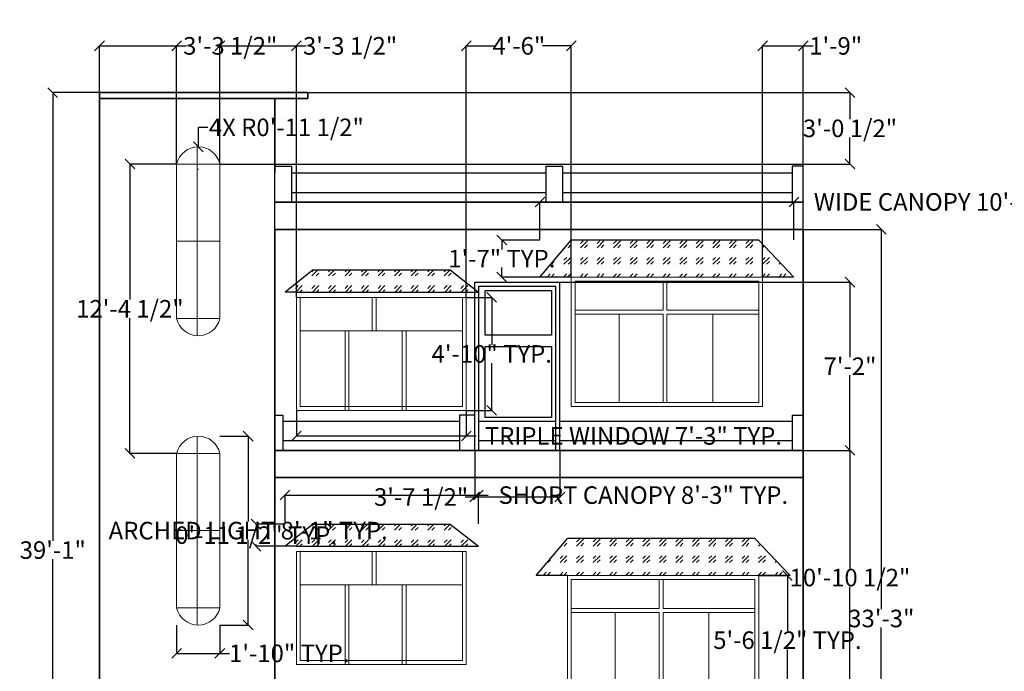
# Model space of a CAD drawing. Units: inches. Extents: x -19 to 1000, y -122 to 1144.
# Tile 7 of 8: x -19 to 486, y 501 to 835. Entities that reach past the tile are written whole.
import ezdxf

# ---------------------------------------------------------------- set-up
doc = ezdxf.new("R2010")
doc.units = ezdxf.units.IN
doc.header["$MEASUREMENT"] = 0
for name, color, linetype, lineweight in [('A-ANNO-DIMS', 191, 'Continuous', 18), ('A-ELEV', 4, 'Continuous', 35), ('A-ELEV-DOOR', 2, 'Continuous', 25), ('A-ELEV-GLAZ', 3, 'Continuous', 18), ('A-ELEV-PATT', 8, 'Continuous', 13), ('A-ELEV-RAIL', 4, 'Continuous', 25), ('A-ELEV-SHAD', 4, 'Continuous', 25)]:
    doc.layers.add(name, color=color, linetype=linetype, lineweight=lineweight)
doc.styles.get("Standard").update_dxf_attribs({"font": 'arial.ttf'})
doc.dimstyles.get("Standard").update_dxf_attribs({"dimtxt": 9, "dimasz": 5, "dimexe": 0.18, "dimexo": 0.0625, "dimgap": 0.09, "dimtad": 0, "dimtih": 1, "dimtoh": 1, "dimdec": 0, "dimzin": 0, "dimdsep": 46, "dimlunit": 3, "dimtxsty": 'Standard', "dimblk": 'OBLIQUE', "dimcen": 0.09, "dimadec": 0, "dimazin": 0, "dimtfac": 1, "dimtdec": 0, "dimtofl": 0, "dimtmove": 0, "dimatfit": 3, "dimfxl": 1, "dimtolj": 1, "dimtzin": 0, "dimarcsym": 0})

# ---------------------------------------------------------------- blocks, each defined once
blk = doc.blocks.new('_Oblique')
at = {"color": 0, "linetype": 'ByBlock', "lineweight": -2}
blk.add_line((-0.5, -0.5), (0.5, 0.5), dxfattribs=at)
blk = doc.blocks.new('*D9')
at = {"layer": 'A-ANNO-DIMS', "color": 0, "lineweight": -2, "transparency": 16777216}
for p, q in [((382.7, 727.13), (422.85, 727.13)), ((422.67, 727.13), (422.67, 532.32)), ((422.67, 328.13), (422.67, 522.95)), ((382.7, 328.13), (422.85, 328.13))]:
    blk.add_line(p, q, dxfattribs=at)
at = {"layer": 'Defpoints', "color": 0, "transparency": 16777216}
for p in [(382.64, 727.13), (422.67, 727.13), (382.64, 328.13)]:
    blk.add_point(p, dxfattribs=at)
at = {"layer": 'A-ANNO-DIMS', "color": 0, "lineweight": -2, "transparency": 16777216, "xscale": 5, "yscale": 5, "zscale": 5}
for p, rotation in [((422.67, 727.13), 90), ((422.67, 328.13), 270)]:
    blk.add_blockref('_Oblique', p, dxfattribs=dict(at, rotation=rotation))
at = {"layer": 'A-ANNO-DIMS', "color": 0, "transparency": 16777216, "insert": (422.67, 527.63), "char_height": 9, "attachment_point": 5}
blk.add_mtext('\\A1;33\'-3"', dxfattribs=at)
blk = doc.blocks.new('WINDOW-ELEV-WIDE')
for p, q in [((47.06, 49.36), (47.06, 64.32)), ((49.06, 49.36), (49.06, 64.32)), ((2, 49.36), (47.06, 49.36)), ((2, 47.36), (47.06, 47.36)), ((24.53, 47.36), (24.53, 2)), ((47.06, 2), (47.06, 47.36)), ((49.06, 49.36), (96.11, 49.36)), ((49.06, 2), (49.06, 47.36)), ((49.06, 47.36), (96.11, 47.36)), ((72.58, 47.36), (72.58, 2))]:
    blk.add_line(p, q)
for points in [[(98.11, 0), (0, 0), (0, 66.32), (98.11, 66.32)], [(96.11, 2), (2, 2), (2, 64.32), (96.11, 64.32)]]:
    blk.add_lwpolyline(points, close=True)
blk = doc.blocks.new('WINDOW-ELEV-TRIPLE')
for p, q in [((0, 57.95), (87.14, 57.95)), ((38.95, 40.87), (38.95, 57.95)), ((40.95, 40.87), (40.95, 57.95)), ((2, 40.87), (85.14, 40.87)), ((24.97, 0), (24.97, 40.87)), ((26.97, 0), (26.97, 40.87)), ((54.23, 0), (54.23, 40.87)), ((56.23, 0), (56.23, 40.87))]:
    blk.add_line(p, q)
for points in [[(87.14, 57.95), (87.14, 0), (0, 0), (0, 57.95)], [(85.14, 57.95), (85.14, 2), (2, 2), (2, 57.95)]]:
    blk.add_lwpolyline(points)
blk = doc.blocks.new('WINDOW-ELEV-ARCHED')
for p, q in [((10.56, 0.01), (10.56, 96.82)), ((0, 8.85), (0, 87.99)), ((0, 87.99), (22.2, 87.99)), ((22.2, 8.85), (22.2, 87.99)), ((0, 48.42), (22.2, 48.42)), ((0, 8.85), (22.2, 8.85))]:
    blk.add_line(p, q)
for centre, start, end in [((11.1, 85.45), 12.876, 167.124), ((11.1, 11.39), 192.876, 347.124)]:
    blk.add_arc(centre, 11.39, start, end)
blk = doc.blocks.new('CANOPY-WIDE-ELEV')
for p, q in [((0, 0), (16.1, 19.04)), ((112.22, 19.04), (16.1, 19.04)), ((130.32, 0), (112.22, 19.04)), ((16.1, 0), (0, 0)), ((130.32, 0), (114.22, 0))]:
    blk.add_line(p, q)
blk = doc.blocks.new('CANOPY-SHORT-ELEV')
for p, q in [((14.47, 11.31), (0, 0)), ((14.47, 11.31), (84.74, 11.31)), ((84.74, 11.31), (99.21, 0)), ((5.84, 0), (0, 0)), ((92.97, 0), (99.21, 0))]:
    blk.add_line(p, q)
blk.add_lwpolyline([(5.84, 0), (92.97, 0)])
blk = doc.blocks.new('*D74')
at = {"layer": 'A-ANNO-DIMS', "color": 0, "lineweight": -2, "transparency": 16777216}
for p, q in [((359.84, 549.66), (374.68, 549.66)), ((374.5, 549.66), (374.5, 521.25)), ((374.5, 483.35), (374.5, 511.76)), ((359.84, 483.35), (374.68, 483.35))]:
    blk.add_line(p, q, dxfattribs=at)
at = {"layer": 'Defpoints', "color": 0, "transparency": 16777216}
for p in [(359.78, 549.66), (374.5, 549.66), (359.78, 483.35)]:
    blk.add_point(p, dxfattribs=at)
at = {"layer": 'A-ANNO-DIMS', "color": 0, "lineweight": -2, "transparency": 16777216, "xscale": 5, "yscale": 5, "zscale": 5}
for p, rotation in [((374.5, 549.66), 90), ((374.5, 483.35), 270)]:
    blk.add_blockref('_Oblique', p, dxfattribs=dict(at, rotation=rotation))
at = {"layer": 'A-ANNO-DIMS', "color": 0, "transparency": 16777216, "insert": (374.5, 516.51), "char_height": 9, "attachment_point": 5}
blk.add_mtext('\\A1;5\'-6 1/2" TYP.', dxfattribs=at)
blk = doc.blocks.new('*D75')
at = {"layer": 'A-ANNO-DIMS', "color": 0, "lineweight": -2, "transparency": 16777216}
for p, q in [((122.65, 634.26), (122.65, 621.07)), ((209.79, 634.26), (209.79, 621.07)), ((122.65, 621.25), (209.79, 621.25)), ((209.79, 621.25), (214.79, 621.25))]:
    blk.add_line(p, q, dxfattribs=at)
at = {"layer": 'Defpoints', "color": 0, "transparency": 16777216}
for p in [(122.65, 634.32), (209.79, 634.32), (209.79, 621.25)]:
    blk.add_point(p, dxfattribs=at)
at = {"layer": 'A-ANNO-DIMS', "color": 0, "lineweight": -2, "transparency": 16777216, "xscale": 5, "yscale": 5, "zscale": 5, "rotation": 180}
blk.add_blockref('_Oblique', (122.65, 621.25), dxfattribs=at)
at = {"layer": 'A-ANNO-DIMS', "color": 0, "lineweight": -2, "transparency": 16777216, "xscale": 5, "yscale": 5, "zscale": 5}
blk.add_blockref('_Oblique', (209.79, 621.25), dxfattribs=at)
at = {"layer": 'A-ANNO-DIMS', "color": 0, "transparency": 16777216, "insert": (295.51, 621.25), "char_height": 9, "attachment_point": 5}
blk.add_mtext('\\A1;TRIPLE WINDOW 7\'-3" TYP.', dxfattribs=at)
blk = doc.blocks.new('*D76')
at = {"layer": 'A-ANNO-DIMS', "color": 0, "lineweight": -2, "transparency": 16777216}
for p, q in [((209.86, 692.27), (223.04, 692.27)), ((222.86, 692.27), (222.86, 667.98)), ((222.86, 634.32), (222.86, 658.61)), ((209.86, 634.32), (223.04, 634.32))]:
    blk.add_line(p, q, dxfattribs=at)
at = {"layer": 'Defpoints', "color": 0, "transparency": 16777216}
for p in [(209.79, 692.27), (222.86, 692.27), (209.79, 634.32)]:
    blk.add_point(p, dxfattribs=at)
at = {"layer": 'A-ANNO-DIMS', "color": 0, "lineweight": -2, "transparency": 16777216, "xscale": 5, "yscale": 5, "zscale": 5}
for p, rotation in [((222.86, 692.27), 90), ((222.86, 634.32), 270)]:
    blk.add_blockref('_Oblique', p, dxfattribs=dict(at, rotation=rotation))
at = {"layer": 'A-ANNO-DIMS', "color": 0, "transparency": 16777216, "insert": (222.86, 663.3), "char_height": 9, "attachment_point": 5}
blk.add_mtext('\\A1;4\'-10" TYP.', dxfattribs=at)
blk = doc.blocks.new('*D77')
at = {"layer": 'A-ANNO-DIMS', "color": 0, "lineweight": -2, "transparency": 16777216}
for p, q in [((83.46, 621.11), (98.11, 621.11)), ((97.93, 621.11), (97.93, 577.43)), ((97.93, 524.27), (97.93, 567.94)), ((83.46, 524.27), (98.11, 524.27))]:
    blk.add_line(p, q, dxfattribs=at)
at = {"layer": 'Defpoints', "color": 0, "transparency": 16777216}
for p in [(83.4, 621.11), (97.93, 621.11), (83.4, 524.27)]:
    blk.add_point(p, dxfattribs=at)
at = {"layer": 'A-ANNO-DIMS', "color": 0, "lineweight": -2, "transparency": 16777216, "xscale": 5, "yscale": 5, "zscale": 5}
for p, rotation in [((97.93, 621.11), 90), ((97.93, 524.27), 270)]:
    blk.add_blockref('_Oblique', p, dxfattribs=dict(at, rotation=rotation))
at = {"layer": 'A-ANNO-DIMS', "color": 0, "transparency": 16777216, "insert": (97.93, 572.69), "char_height": 9, "attachment_point": 5}
blk.add_mtext('\\A1;ARCHED LIGHT 8\'-1" TYP.', dxfattribs=at)
blk = doc.blocks.new('*D78')
at = {"layer": 'A-ANNO-DIMS', "color": 0, "lineweight": -2, "transparency": 16777216}
for p, q in [((61.2, 524.21), (61.2, 509.56)), ((83.4, 524.21), (83.4, 509.56)), ((61.2, 509.74), (83.4, 509.74)), ((83.4, 509.74), (88.4, 509.74))]:
    blk.add_line(p, q, dxfattribs=at)
at = {"layer": 'Defpoints', "color": 0, "transparency": 16777216}
for p in [(61.2, 524.27), (83.4, 524.27), (83.4, 509.74)]:
    blk.add_point(p, dxfattribs=at)
at = {"layer": 'A-ANNO-DIMS', "color": 0, "lineweight": -2, "transparency": 16777216, "xscale": 5, "yscale": 5, "zscale": 5, "rotation": 180}
blk.add_blockref('_Oblique', (61.2, 509.74), dxfattribs=at)
at = {"layer": 'A-ANNO-DIMS', "color": 0, "lineweight": -2, "transparency": 16777216, "xscale": 5, "yscale": 5, "zscale": 5}
blk.add_blockref('_Oblique', (83.4, 509.74), dxfattribs=at)
at = {"layer": 'A-ANNO-DIMS', "color": 0, "transparency": 16777216, "insert": (118.99, 509.74), "char_height": 9, "attachment_point": 5}
blk.add_mtext('\\A1;1\'-10" TYP.', dxfattribs=at)
blk = doc.blocks.new('*D79')
at = {"layer": 'A-ANNO-DIMS', "color": 0, "lineweight": -2, "transparency": 16777216}
for p, q in [((247.56, 721.74), (247.56, 741.41)), ((247.56, 741.23), (377.88, 741.23)), ((377.88, 721.74), (377.88, 741.41)), ((377.88, 741.23), (382.88, 741.23))]:
    blk.add_line(p, q, dxfattribs=at)
at = {"layer": 'Defpoints', "color": 0, "transparency": 16777216}
for p in [(377.88, 741.23), (247.56, 721.68), (377.88, 721.68)]:
    blk.add_point(p, dxfattribs=at)
at = {"layer": 'A-ANNO-DIMS', "color": 0, "lineweight": -2, "transparency": 16777216, "xscale": 5, "yscale": 5, "zscale": 5, "rotation": 180}
blk.add_blockref('_Oblique', (247.56, 741.23), dxfattribs=at)
at = {"layer": 'A-ANNO-DIMS', "color": 0, "lineweight": -2, "transparency": 16777216, "xscale": 5, "yscale": 5, "zscale": 5}
blk.add_blockref('_Oblique', (377.88, 741.23), dxfattribs=at)
at = {"layer": 'A-ANNO-DIMS', "color": 0, "transparency": 16777216, "insert": (474.52, 741.23), "char_height": 9, "attachment_point": 5}
blk.add_mtext('\\A1;WIDE CANOPY 10\'-10 1/2" TYP.', dxfattribs=at)
blk = doc.blocks.new('*D80')
at = {"layer": 'A-ANNO-DIMS', "color": 0, "lineweight": -2, "transparency": 16777216}
for p, q in [((247.5, 721.68), (227.83, 721.68)), ((228.01, 721.68), (228.01, 716.77)), ((228.01, 702.64), (228.01, 707.55)), ((247.5, 702.64), (227.83, 702.64))]:
    blk.add_line(p, q, dxfattribs=at)
at = {"layer": 'Defpoints', "color": 0, "transparency": 16777216}
for p in [(228.01, 721.68), (247.56, 721.68), (247.56, 702.64)]:
    blk.add_point(p, dxfattribs=at)
at = {"layer": 'A-ANNO-DIMS', "color": 0, "lineweight": -2, "transparency": 16777216, "xscale": 5, "yscale": 5, "zscale": 5}
for p, rotation in [((228.01, 721.68), 90), ((228.01, 702.64), 270)]:
    blk.add_blockref('_Oblique', p, dxfattribs=dict(at, rotation=rotation))
at = {"layer": 'A-ANNO-DIMS', "color": 0, "transparency": 16777216, "insert": (228.01, 712.16), "char_height": 9, "attachment_point": 5}
blk.add_mtext('\\A1;1\'-7" TYP.', dxfattribs=at)
blk = doc.blocks.new('*D81')
at = {"layer": 'A-ANNO-DIMS', "color": 0, "lineweight": -2, "transparency": 16777216}
for p, q in [((116.82, 576.08), (116.82, 591.08)), ((116.82, 590.9), (216.03, 590.9)), ((216.03, 576.08), (216.03, 591.08)), ((216.03, 590.9), (221.03, 590.9))]:
    blk.add_line(p, q, dxfattribs=at)
at = {"layer": 'Defpoints', "color": 0, "transparency": 16777216}
for p in [(216.03, 590.9), (116.82, 576.01), (216.03, 576.01)]:
    blk.add_point(p, dxfattribs=at)
at = {"layer": 'A-ANNO-DIMS', "color": 0, "lineweight": -2, "transparency": 16777216, "xscale": 5, "yscale": 5, "zscale": 5, "rotation": 180}
blk.add_blockref('_Oblique', (116.82, 590.9), dxfattribs=at)
at = {"layer": 'A-ANNO-DIMS', "color": 0, "lineweight": -2, "transparency": 16777216, "xscale": 5, "yscale": 5, "zscale": 5}
blk.add_blockref('_Oblique', (216.03, 590.9), dxfattribs=at)
at = {"layer": 'A-ANNO-DIMS', "color": 0, "transparency": 16777216, "insert": (300.57, 590.9), "char_height": 9, "attachment_point": 5}
blk.add_mtext('\\A1;SHORT CANOPY 8\'-3" TYP.', dxfattribs=at)
blk = doc.blocks.new('*D82')
at = {"layer": 'A-ANNO-DIMS', "color": 0, "lineweight": -2, "transparency": 16777216}
for p, q in [((116.76, 576.01), (101.76, 576.01)), ((101.94, 576.01), (101.94, 575.1)), ((116.76, 564.71), (101.76, 564.71)), ((101.94, 564.71), (101.94, 565.62))]:
    blk.add_line(p, q, dxfattribs=at)
at = {"layer": 'Defpoints', "color": 0, "transparency": 16777216}
for p in [(101.94, 576.01), (116.82, 576.01), (116.82, 564.71)]:
    blk.add_point(p, dxfattribs=at)
at = {"layer": 'A-ANNO-DIMS', "color": 0, "lineweight": -2, "transparency": 16777216, "xscale": 5, "yscale": 5, "zscale": 5}
for p, rotation in [((101.94, 576.01), 90), ((101.94, 564.71), 270)]:
    blk.add_blockref('_Oblique', p, dxfattribs=dict(at, rotation=rotation))
at = {"layer": 'A-ANNO-DIMS', "color": 0, "transparency": 16777216, "insert": (101.94, 570.36), "char_height": 9, "attachment_point": 5}
blk.add_mtext('\\A1;0\'-11 1/2" TYP.', dxfattribs=at)
blk = doc.blocks.new('*D112')
at = {"layer": 'A-ANNO-DIMS', "color": 0, "lineweight": -2, "transparency": 16777216}
for p, q in [((21.58, 797.3), (-2.49, 797.3)), ((-2.31, 797.3), (-2.31, 567.4)), ((-2.31, 328.13), (-2.31, 558.03)), ((21.58, 328.13), (-2.49, 328.13))]:
    blk.add_line(p, q, dxfattribs=at)
at = {"layer": 'Defpoints', "color": 0, "transparency": 16777216}
for p in [(-2.31, 797.3), (21.64, 797.3), (21.64, 328.13)]:
    blk.add_point(p, dxfattribs=at)
at = {"layer": 'A-ANNO-DIMS', "color": 0, "lineweight": -2, "transparency": 16777216, "xscale": 5, "yscale": 5, "zscale": 5}
for p, rotation in [((-2.31, 797.3), 90), ((-2.31, 328.13), 270)]:
    blk.add_blockref('_Oblique', p, dxfattribs=dict(at, rotation=rotation))
at = {"layer": 'A-ANNO-DIMS', "color": 0, "transparency": 16777216, "insert": (-2.31, 562.72), "char_height": 9, "attachment_point": 5}
blk.add_mtext('\\A1;39\'-1"', dxfattribs=at)
blk = doc.blocks.new('*D119')
at = {"layer": 'A-ANNO-DIMS', "color": 0, "lineweight": -2, "transparency": 16777216}
for p, q in [((61.14, 760.62), (37.07, 760.62)), ((37.25, 760.62), (37.25, 691.18)), ((37.25, 612.26), (37.25, 681.69)), ((61.14, 612.26), (37.07, 612.26))]:
    blk.add_line(p, q, dxfattribs=at)
at = {"layer": 'Defpoints', "color": 0, "transparency": 16777216}
for p in [(37.25, 760.62), (61.2, 760.62), (61.2, 612.26)]:
    blk.add_point(p, dxfattribs=at)
at = {"layer": 'A-ANNO-DIMS', "color": 0, "lineweight": -2, "transparency": 16777216, "xscale": 5, "yscale": 5, "zscale": 5}
for p, rotation in [((37.25, 760.62), 90), ((37.25, 612.26), 270)]:
    blk.add_blockref('_Oblique', p, dxfattribs=dict(at, rotation=rotation))
at = {"layer": 'A-ANNO-DIMS', "color": 0, "transparency": 16777216, "insert": (37.25, 686.44), "char_height": 9, "attachment_point": 5}
blk.add_mtext('\\A1;12\'-4 1/2"', dxfattribs=at)
blk = doc.blocks.new('*D120')
at = {"layer": 'A-ANNO-DIMS', "color": 0, "lineweight": -2, "transparency": 16777216}
for p, q in [((128.58, 797.3), (406.77, 797.3)), ((406.59, 797.3), (406.59, 783.7)), ((406.59, 760.62), (406.59, 774.21)), ((83.46, 760.62), (406.77, 760.62))]:
    blk.add_line(p, q, dxfattribs=at)
at = {"layer": 'Defpoints', "color": 0, "transparency": 16777216}
for p in [(128.51, 797.3), (406.59, 797.3), (83.4, 760.62)]:
    blk.add_point(p, dxfattribs=at)
at = {"layer": 'A-ANNO-DIMS', "color": 0, "lineweight": -2, "transparency": 16777216, "xscale": 5, "yscale": 5, "zscale": 5}
for p, rotation in [((406.59, 797.3), 90), ((406.59, 760.62), 270)]:
    blk.add_blockref('_Oblique', p, dxfattribs=dict(at, rotation=rotation))
at = {"layer": 'A-ANNO-DIMS', "color": 0, "transparency": 16777216, "insert": (406.59, 778.96), "char_height": 9, "attachment_point": 5}
blk.add_mtext('\\A1;3\'-0 1/2"', dxfattribs=at)
blk = doc.blocks.new('*D122')
at = {"layer": 'A-ANNO-DIMS', "color": 0, "lineweight": -2, "transparency": 16777216}
for p, q in [((382.7, 613.85), (406.77, 613.85)), ((406.59, 613.85), (406.59, 553.34)), ((406.59, 483.35), (406.59, 543.86)), ((359.84, 483.35), (406.77, 483.35))]:
    blk.add_line(p, q, dxfattribs=at)
at = {"layer": 'Defpoints', "color": 0, "transparency": 16777216}
for p in [(382.64, 613.85), (406.59, 613.85), (359.78, 483.35)]:
    blk.add_point(p, dxfattribs=at)
at = {"layer": 'A-ANNO-DIMS', "color": 0, "lineweight": -2, "transparency": 16777216, "xscale": 5, "yscale": 5, "zscale": 5}
for p, rotation in [((406.59, 613.85), 90), ((406.59, 483.35), 270)]:
    blk.add_blockref('_Oblique', p, dxfattribs=dict(at, rotation=rotation))
at = {"layer": 'A-ANNO-DIMS', "color": 0, "transparency": 16777216, "insert": (406.59, 548.6), "char_height": 9, "attachment_point": 5}
blk.add_mtext('\\A1;10\'-10 1/2"', dxfattribs=at)
blk = doc.blocks.new('*D123')
at = {"layer": 'A-ANNO-DIMS', "color": 0, "lineweight": -2, "transparency": 16777216}
for p, q in [((209.79, 692.34), (209.79, 821.43)), ((209.79, 821.25), (224.5, 821.25)), ((263.67, 821.25), (248.96, 821.25)), ((263.67, 702.7), (263.67, 821.43))]:
    blk.add_line(p, q, dxfattribs=at)
at = {"layer": 'Defpoints', "color": 0, "transparency": 16777216}
for p in [(263.67, 821.25), (263.67, 702.64), (209.79, 692.27)]:
    blk.add_point(p, dxfattribs=at)
at = {"layer": 'A-ANNO-DIMS', "color": 0, "lineweight": -2, "transparency": 16777216, "xscale": 5, "yscale": 5, "zscale": 5, "rotation": 180}
blk.add_blockref('_Oblique', (209.79, 821.25), dxfattribs=at)
at = {"layer": 'A-ANNO-DIMS', "color": 0, "lineweight": -2, "transparency": 16777216, "xscale": 5, "yscale": 5, "zscale": 5}
blk.add_blockref('_Oblique', (263.67, 821.25), dxfattribs=at)
at = {"layer": 'A-ANNO-DIMS', "color": 0, "transparency": 16777216, "insert": (236.73, 821.25), "char_height": 9, "attachment_point": 5}
blk.add_mtext('\\A1;4\'-6"', dxfattribs=at)
blk = doc.blocks.new('*D124')
at = {"layer": 'A-ANNO-DIMS', "color": 0, "lineweight": -2, "transparency": 16777216}
for p, q in [((361.78, 702.7), (361.78, 821.43)), ((361.78, 821.25), (382.64, 821.25)), ((382.64, 727.2), (382.64, 821.43)), ((382.64, 821.25), (387.64, 821.25))]:
    blk.add_line(p, q, dxfattribs=at)
at = {"layer": 'Defpoints', "color": 0, "transparency": 16777216}
for p in [(382.64, 821.25), (382.64, 727.13), (361.78, 702.64)]:
    blk.add_point(p, dxfattribs=at)
at = {"layer": 'A-ANNO-DIMS', "color": 0, "lineweight": -2, "transparency": 16777216, "xscale": 5, "yscale": 5, "zscale": 5, "rotation": 180}
blk.add_blockref('_Oblique', (361.78, 821.25), dxfattribs=at)
at = {"layer": 'A-ANNO-DIMS', "color": 0, "lineweight": -2, "transparency": 16777216, "xscale": 5, "yscale": 5, "zscale": 5}
blk.add_blockref('_Oblique', (382.64, 821.25), dxfattribs=at)
at = {"layer": 'A-ANNO-DIMS', "color": 0, "transparency": 16777216, "insert": (399.27, 821.25), "char_height": 9, "attachment_point": 5}
blk.add_mtext('\\A1;1\'-9"', dxfattribs=at)
blk = doc.blocks.new('*D125')
at = {"layer": 'A-ANNO-DIMS', "color": 0, "lineweight": -2, "transparency": 16777216}
for p, q in [((21.64, 797.36), (21.64, 821.43)), ((21.64, 821.25), (61.2, 821.25)), ((61.2, 760.68), (61.2, 821.43)), ((61.2, 821.25), (66.2, 821.25))]:
    blk.add_line(p, q, dxfattribs=at)
at = {"layer": 'Defpoints', "color": 0, "transparency": 16777216}
for p in [(61.2, 821.25), (21.64, 797.3), (61.2, 760.62)]:
    blk.add_point(p, dxfattribs=at)
at = {"layer": 'A-ANNO-DIMS', "color": 0, "lineweight": -2, "transparency": 16777216, "xscale": 5, "yscale": 5, "zscale": 5, "rotation": 180}
blk.add_blockref('_Oblique', (21.64, 821.25), dxfattribs=at)
at = {"layer": 'A-ANNO-DIMS', "color": 0, "lineweight": -2, "transparency": 16777216, "xscale": 5, "yscale": 5, "zscale": 5}
blk.add_blockref('_Oblique', (61.2, 821.25), dxfattribs=at)
at = {"layer": 'A-ANNO-DIMS', "color": 0, "transparency": 16777216, "insert": (88.73, 821.25), "char_height": 9, "attachment_point": 5}
blk.add_mtext('\\A1;3\'-3 1/2"', dxfattribs=at)
blk = doc.blocks.new('*D126')
at = {"layer": 'A-ANNO-DIMS', "color": 0, "lineweight": -2, "transparency": 16777216}
for p, q in [((83.4, 760.68), (83.4, 821.43)), ((83.4, 821.25), (122.65, 821.25)), ((122.65, 692.34), (122.65, 821.43)), ((122.65, 821.25), (127.65, 821.25))]:
    blk.add_line(p, q, dxfattribs=at)
at = {"layer": 'Defpoints', "color": 0, "transparency": 16777216}
for p in [(122.65, 821.25), (83.4, 760.62), (122.65, 692.27)]:
    blk.add_point(p, dxfattribs=at)
at = {"layer": 'A-ANNO-DIMS', "color": 0, "lineweight": -2, "transparency": 16777216, "xscale": 5, "yscale": 5, "zscale": 5, "rotation": 180}
blk.add_blockref('_Oblique', (83.4, 821.25), dxfattribs=at)
at = {"layer": 'A-ANNO-DIMS', "color": 0, "lineweight": -2, "transparency": 16777216, "xscale": 5, "yscale": 5, "zscale": 5}
blk.add_blockref('_Oblique', (122.65, 821.25), dxfattribs=at)
at = {"layer": 'A-ANNO-DIMS', "color": 0, "transparency": 16777216, "insert": (150.19, 821.25), "char_height": 9, "attachment_point": 5}
blk.add_mtext('\\A1;3\'-3 1/2"', dxfattribs=at)
blk = doc.blocks.new('*D127')
at = {"layer": 'A-ANNO-DIMS', "color": 0, "lineweight": -2, "transparency": 16777216}
for p, q in [((214.15, 613.79), (214.15, 589.72)), ((257.78, 613.79), (257.78, 589.72)), ((214.15, 589.9), (209.15, 589.9)), ((257.78, 589.9), (214.15, 589.9))]:
    blk.add_line(p, q, dxfattribs=at)
at = {"layer": 'Defpoints', "color": 0, "transparency": 16777216}
for p in [(214.15, 613.85), (257.78, 613.85), (214.15, 589.9)]:
    blk.add_point(p, dxfattribs=at)
at = {"layer": 'A-ANNO-DIMS', "color": 0, "lineweight": -2, "transparency": 16777216, "xscale": 5, "yscale": 5, "zscale": 5, "rotation": 180}
blk.add_blockref('_Oblique', (214.15, 589.9), dxfattribs=at)
at = {"layer": 'A-ANNO-DIMS', "color": 0, "lineweight": -2, "transparency": 16777216, "xscale": 5, "yscale": 5, "zscale": 5}
blk.add_blockref('_Oblique', (257.78, 589.9), dxfattribs=at)
at = {"layer": 'A-ANNO-DIMS', "color": 0, "transparency": 16777216, "insert": (186.62, 589.9), "char_height": 9, "attachment_point": 5}
blk.add_mtext('\\A1;3\'-7 1/2"', dxfattribs=at)
blk = doc.blocks.new('*D128')
at = {"layer": 'A-ANNO-DIMS', "color": 0, "lineweight": -2, "transparency": 16777216}
for p, q in [((257.85, 700.08), (406.77, 700.08)), ((406.59, 700.08), (406.59, 661.58)), ((406.59, 613.85), (406.59, 652.36)), ((382.7, 613.85), (406.77, 613.85))]:
    blk.add_line(p, q, dxfattribs=at)
at = {"layer": 'Defpoints', "color": 0, "transparency": 16777216}
for p in [(257.78, 700.08), (406.59, 700.08), (382.64, 613.85)]:
    blk.add_point(p, dxfattribs=at)
at = {"layer": 'A-ANNO-DIMS', "color": 0, "lineweight": -2, "transparency": 16777216, "xscale": 5, "yscale": 5, "zscale": 5}
for p, rotation in [((406.59, 700.08), 90), ((406.59, 613.85), 270)]:
    blk.add_blockref('_Oblique', p, dxfattribs=dict(at, rotation=rotation))
at = {"layer": 'A-ANNO-DIMS', "color": 0, "transparency": 16777216, "insert": (406.59, 656.97), "char_height": 9, "attachment_point": 5}
blk.add_mtext('\\A1;7\'-2"', dxfattribs=at)
blk = doc.blocks.new('*D149')
at = {"layer": 'A-ANNO-DIMS', "color": 0, "lineweight": -2, "transparency": 16777216}
for p, q in [((77.3, 779.47), (72.3, 779.47)), ((72.3, 779.47), (72.3, 769.47)), ((72.21, 758.08), (72.39, 758.08)), ((72.3, 757.99), (72.3, 758.17))]:
    blk.add_line(p, q, dxfattribs=at)
at = {"layer": 'Defpoints', "color": 0, "transparency": 16777216}
for p in [(72.3, 769.47), (72.3, 758.08)]:
    blk.add_point(p, dxfattribs=at)
at = {"layer": 'A-ANNO-DIMS', "color": 0, "lineweight": -2, "transparency": 16777216, "xscale": 5, "yscale": 5, "zscale": 5, "rotation": 269.9991144404323}
blk.add_blockref('_Oblique', (72.3, 769.47), dxfattribs=at)
at = {"layer": 'A-ANNO-DIMS', "color": 0, "transparency": 16777216, "insert": (117.49, 779.47), "char_height": 9, "attachment_point": 5}
blk.add_mtext('\\A1;4X R0\'-11 1/2"', dxfattribs=at)

msp = doc.modelspace()

# ---------------------------------------------------------------- hatches: boundary and pattern name
at = {"layer": 'A-ELEV-PATT'}
h = msp.add_hatch(dxfattribs=at)
h.set_pattern_fill('GOST_GLASS', color=256)
h.set_pattern_definition([(45, (-435.899, -113.8284), (8.48528, 0), [5, -7]), (45, (-433.7775, -113.8284), (8.48528, 0), [2, -10]), (45, (-435.899, -111.707), (8.48528, 0), [2, -10])])
h.paths.add_polyline_path([(359.78, 721.68), (263.67, 721.68), (247.56, 702.64), (263.67, 702.64), (361.78, 702.64), (377.88, 702.64)])
h = msp.add_hatch(dxfattribs=at)
h.set_pattern_fill('GOST_GLASS', color=256)
h.set_pattern_definition([(45, (-437.899, -187.694), (8.48528, 0), [5, -7]), (45, (-435.7775, -187.694), (8.48528, 0), [2, -10]), (45, (-437.899, -185.5725), (8.48528, 0), [2, -10])])
h.paths.add_polyline_path([(201.56, 706.33), (131.29, 706.33), (116.82, 695.02), (122.65, 695.02), (209.79, 695.02), (216.03, 695.02)])
h = msp.add_hatch(dxfattribs=at)
h.set_pattern_fill('GOST_GLASS', color=256)
h.set_pattern_definition([(45, (-437.899, -318.008), (8.48528, 0), [5, -7]), (45, (-435.7775, -318.008), (8.48528, 0), [2, -10]), (45, (-437.899, -315.8866), (8.48528, 0), [2, -10])])
h.paths.add_polyline_path([(201.56, 576.01), (131.29, 576.01), (116.82, 564.71), (122.65, 564.71), (209.79, 564.71), (216.03, 564.71)])
h = msp.add_hatch(dxfattribs=at)
h.set_pattern_fill('GOST_GLASS', color=256)
h.set_pattern_definition([(45, (-437.899, -266.802), (8.48528, 0), [5, -7]), (45, (-435.7775, -266.802), (8.48528, 0), [2, -10]), (45, (-437.899, -264.681), (8.48528, 0), [2, -10])])
h.paths.add_polyline_path([(357.78, 568.7), (261.67, 568.7), (245.56, 549.66), (261.67, 549.66), (359.78, 549.66), (375.88, 549.66)])

# ---------------------------------------------------------------- linework, layer by layer
at = {"layer": 'A-ELEV'}
for p, q in [((21.64, 756.13), (21.64, 797.3)), ((21.64, 797.3), (128.51, 797.3)), ((21.64, 794.3), (128.51, 794.3)), ((111.64, 756.13), (111.64, 794.3)), ((128.51, 794.3), (128.51, 797.3)), ((21.64, 727.13), (21.64, 756.13)), ((111.64, 741.13), (382.64, 741.13)), ((21.64, 328.13), (21.64, 727.13)), ((111.64, 364.13), (111.64, 727.13)), ((382.64, 727.13), (111.64, 727.13)), ((111.64, 727.13), (382.64, 727.13)), ((382.64, 328.13), (382.64, 727.13)), ((382.64, 328.13), (382.64, 727.13)), ((111.64, 613.85), (382.64, 613.85)), ((111.64, 599.85), (382.64, 599.85))]:
    msp.add_line(p, q, dxfattribs=at)
at = {"layer": 'A-ELEV-DOOR'}
for p, q in [((214.15, 613.85), (214.15, 700.08)), ((214.15, 700.08), (257.78, 700.08)), ((216.15, 698.08), (255.78, 698.08)), ((216.15, 613.85), (216.15, 698.08)), ((255.78, 613.85), (255.78, 698.08)), ((257.78, 613.85), (257.78, 700.08))]:
    msp.add_line(p, q, dxfattribs=at)
for points in [[(253.44, 672.83), (219.55, 672.83), (219.55, 695.77), (253.44, 695.77)], [(219.55, 667.1), (253.44, 667.1), (253.44, 630.64), (219.55, 630.64)]]:
    msp.add_lwpolyline(points, close=True, dxfattribs=at)
at = {"layer": 'A-ELEV-RAIL'}
for p, q in [((111.64, 727.13), (111.64, 759.6)), ((111.64, 759.6), (120.08, 759.6)), ((120.08, 759.6), (120.08, 741.13)), ((250.56, 759.6), (250.56, 741.13)), ((250.56, 759.6), (259.17, 759.6)), ((259.17, 759.6), (259.17, 741.13)), ((382.64, 759.6), (376.93, 759.6)), ((376.93, 759.6), (376.93, 741.13)), ((382.64, 727.13), (382.64, 759.6)), ((120.08, 756.13), (214.15, 756.13)), ((214.15, 756.13), (250.56, 756.13)), ((259.17, 756.13), (376.93, 756.13)), ((120.08, 746.13), (214.15, 746.13)), ((214.15, 746.13), (250.56, 746.13)), ((259.17, 746.13), (376.93, 746.13)), ((111.64, 631.89), (115.77, 631.89)), ((115.77, 631.89), (115.77, 613.85)), ((214.15, 631.89), (206.28, 631.89)), ((206.28, 631.89), (206.28, 613.85)), ((376.93, 631.89), (382.64, 631.89)), ((376.93, 631.89), (376.93, 613.85)), ((115.77, 628.85), (206.28, 628.85)), ((216.15, 628.85), (253.78, 628.85)), ((216.15, 628.85), (255.78, 628.85)), ((257.78, 628.85), (376.93, 628.85)), ((115.77, 618.85), (206.28, 618.85)), ((216.15, 618.85), (253.78, 618.85)), ((216.15, 618.85), (255.78, 618.85)), ((257.78, 618.85), (376.93, 618.85))]:
    msp.add_line(p, q, dxfattribs=at)

# ---------------------------------------------------------------- block references
at = {"layer": 'A-ELEV-GLAZ'}
for name, p in [('WINDOW-ELEV-ARCHED', (61.2, 672.63)), ('WINDOW-ELEV-WIDE', (263.67, 636.32)), ('WINDOW-ELEV-TRIPLE', (122.65, 634.32)), ('WINDOW-ELEV-ARCHED', (61.2, 524.27)), ('WINDOW-ELEV-TRIPLE', (122.65, 504.01)), ('WINDOW-ELEV-WIDE', (261.67, 483.35))]:
    msp.add_blockref(name, p, dxfattribs=at)
at = {"layer": 'A-ELEV-SHAD'}
for name, p in [('CANOPY-WIDE-ELEV', (247.56, 702.64)), ('CANOPY-SHORT-ELEV', (116.82, 695.02)), ('CANOPY-SHORT-ELEV', (116.82, 564.71)), ('CANOPY-WIDE-ELEV', (245.56, 549.66))]:
    msp.add_blockref(name, p, dxfattribs=at)

# ---------------------------------------------------------------- dimensions: what is measured, and where the dimension line sits
at = {"layer": 'A-ANNO-DIMS'}
for base, p1, p2, picture, middle in [((61.2, 821.25), (21.64, 797.3), (61.2, 760.62), '*D125', (88.73, 821.25)), ((122.6534, 821.2479), (83.4007, 760.6184), (122.6534, 692.2741), '*D126', (150.1881, 821.2479)), ((263.67, 821.25), (209.79, 692.27), (263.67, 702.64), '*D123', (236.73, 821.25)), ((382.64, 821.25), (361.78, 702.64), (382.64, 727.13), '*D124', (399.27, 821.25))]:
    dim = msp.add_linear_dim(base=base, p1=p1, p2=p2, dimstyle='Standard', override={"dimdec": 1, "dimlfac": 1, "dimrnd": 0, "dimzin": 1, "dimdsep": 46, "dimlunit": 4, "dimfrac": 2}, dxfattribs=at)
    dim.commit()
    dim.dimension.update_dxf_attribs({"geometry": picture, "text_midpoint": middle})
for base, p1, p2, angle, override, picture, middle in [((-2.31, 797.3), (21.64, 328.13), (21.64, 797.3), 90, {"dimdec": 1, "dimlfac": 1, "dimrnd": 0, "dimzin": 1, "dimdsep": 46, "dimlunit": 4, "dimfrac": 2}, '*D112', (-2.31, 562.72)), ((406.59, 797.3), (83.4, 760.62), (128.51, 797.3), 90, {"dimdec": 1, "dimlfac": 1, "dimrnd": 0, "dimzin": 1, "dimdsep": 46, "dimlunit": 4, "dimfrac": 2}, '*D120', (406.59, 778.96)), ((37.25, 760.62), (61.2, 612.26), (61.2, 760.62), 90, {"dimdec": 1, "dimlfac": 1, "dimrnd": 0, "dimzin": 1, "dimdsep": 46, "dimlunit": 4, "dimfrac": 2}, '*D119', (37.25, 686.44)), ((422.67, 727.13), (382.64, 328.13), (382.64, 727.13), 90, {"dimclrd": 0, "dimclre": 0, "dimclrt": 0}, '*D9', (422.67, 527.63)), ((406.59, 700.08), (382.64, 613.85), (257.78, 700.08), 90, {"dimdec": 1, "dimlfac": 1, "dimrnd": 0, "dimzin": 1, "dimdsep": 46, "dimlunit": 4, "dimfrac": 2}, '*D128', (406.59, 656.97)), ((406.59, 613.85), (359.78, 483.35), (382.64, 613.85), 90, {"dimdec": 1, "dimlfac": 1, "dimrnd": 0, "dimzin": 1, "dimdsep": 46, "dimlunit": 4, "dimfrac": 2}, '*D122', (406.59, 548.6)), ((214.15, 589.9), (257.78, 613.85), (214.15, 613.85), 180, {"dimdec": 1, "dimlfac": 1, "dimrnd": 0, "dimzin": 1, "dimdsep": 46, "dimlunit": 4, "dimfrac": 2}, '*D127', (186.62, 589.9))]:
    dim = msp.add_linear_dim(base=base, p1=p1, p2=p2, angle=angle, dimstyle='Standard', override=override, dxfattribs=at)
    dim.commit()
    dim.dimension.update_dxf_attribs({"geometry": picture, "text_midpoint": middle})
dim = msp.add_radius_dim(center=(72.3, 758.08), mpoint=(72.3, 769.47), text='4X <>', dimstyle='Standard', override={"dimdec": 1, "dimlfac": 1, "dimrnd": 0, "dimzin": 1, "dimdsep": 46, "dimlunit": 4, "dimfrac": 2}, dxfattribs=at)
dim.commit()
dim.dimension.update_dxf_attribs({"geometry": '*D149', "text_midpoint": (117.49, 779.47)})
for base, p1, p2, text, picture, middle in [((377.88, 741.23), (247.56, 721.68), (377.88, 721.68), 'WIDE CANOPY <> TYP.', '*D79', (474.52, 741.23)), ((209.79, 621.25), (122.65, 634.32), (209.79, 634.32), 'TRIPLE WINDOW <> TYP.', '*D75', (295.51, 621.25)), ((216.03, 590.9), (116.82, 576.01), (216.03, 576.01), 'SHORT CANOPY <> TYP.', '*D81', (300.57, 590.9)), ((83.4, 509.74), (61.2, 524.27), (83.4, 524.27), '<> TYP.', '*D78', (118.99, 509.74))]:
    dim = msp.add_linear_dim(base=base, p1=p1, p2=p2, text=text, dimstyle='Standard', override={"dimdec": 1, "dimlfac": 1, "dimrnd": 0, "dimzin": 1, "dimdsep": 46, "dimlunit": 4, "dimfrac": 2}, dxfattribs=at)
    dim.commit()
    dim.dimension.update_dxf_attribs({"geometry": picture, "text_midpoint": middle})
for base, p1, p2, text, picture, middle in [((228.01, 721.68), (247.56, 702.64), (247.56, 721.68), '<> TYP.', '*D80', (228.01, 712.16)), ((222.8634, 692.2741), (209.7926, 634.3207), (209.7926, 692.2741), '<> TYP.', '*D76', (222.8634, 663.2974)), ((97.93, 621.11), (83.4, 524.27), (83.4, 621.11), 'ARCHED LIGHT <> TYP.', '*D77', (97.93, 572.69)), ((101.94, 576.01), (116.82, 564.71), (116.82, 576.01), '<> TYP.', '*D82', (101.94, 570.36)), ((374.5, 549.66), (359.78, 483.35), (359.78, 549.66), '<> TYP.', '*D74', (374.5, 516.51))]:
    dim = msp.add_linear_dim(base=base, p1=p1, p2=p2, angle=90, text=text, dimstyle='Standard', override={"dimdec": 1, "dimlfac": 1, "dimrnd": 0, "dimzin": 1, "dimdsep": 46, "dimlunit": 4, "dimfrac": 2}, dxfattribs=at)
    dim.commit()
    dim.dimension.update_dxf_attribs({"geometry": picture, "text_midpoint": middle})

doc.saveas('drawing.dxf')
